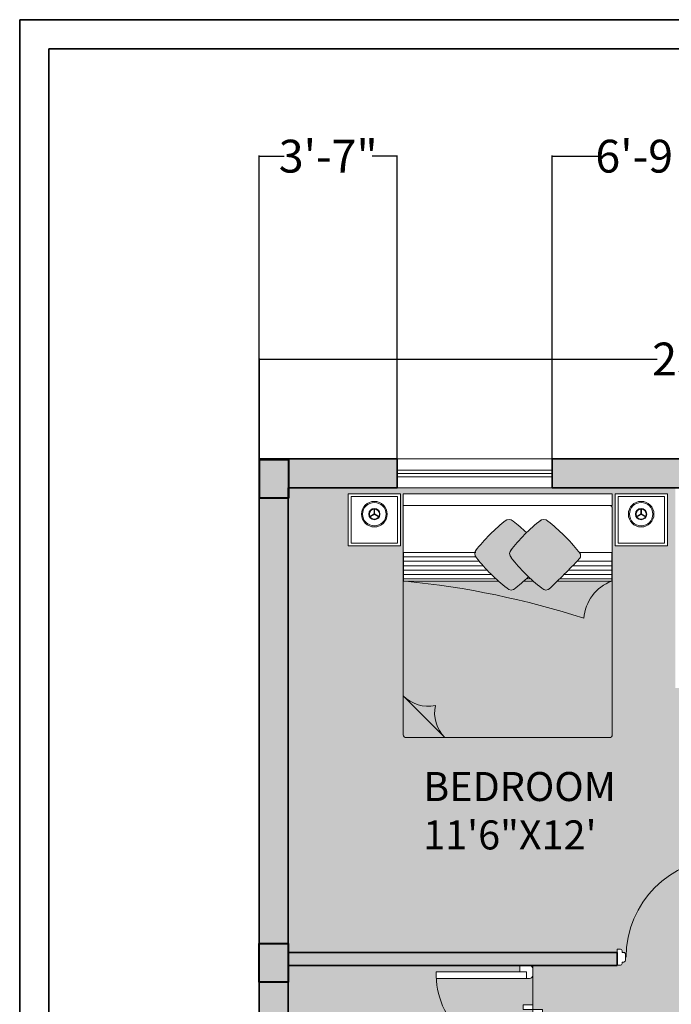
# Model space of a CAD drawing. Units: inches. Extents: x 1077 to 2505, y 1892 to 2728.
# Tile 25 of 26: x 1962 to 2164, y 2423 to 2728. Entities that reach past the tile are written whole.
import ezdxf

# ---------------------------------------------------------------- set-up
doc = ezdxf.new("R2010")
doc.units = ezdxf.units.IN
doc.linetypes.add('ACAD_ISO02W100', pattern=[15, 12, -3])
doc.layers.get('Defpoints').update_dxf_attribs({"color": 220, "linetype": 'ACAD_ISO02W100'})
for name, color, linetype, lineweight in [('00 FURNITURE', 15, 'Continuous', 15), ('A-ANNO-DIMS', 2, 'Continuous', 18), ('A-ANNO-TTLB', 7, 'Continuous', 35), ('A-AREA-IDEN', 7, 'Continuous', 18), ('A-COLS', 7, 'Continuous', 40), ('A-DOOR', 4, 'Continuous', 18), ('A-WALL-PATT', 7, 'Continuous', 9), ('A_FUR 1', 5, 'Continuous', 5), ('WALL', 7, 'Continuous', 35), ('WINDOW', 160, 'Continuous', 13)]:
    doc.layers.add(name, color=color, linetype=linetype, lineweight=lineweight)
doc.layers.add('A-FLOR-PATT', color=254, linetype='Continuous', lineweight=9, true_color=0xd7ebd2)
doc.layers.add('A-FURN-PATT', color=177, linetype='Continuous', lineweight=9, true_color=0x293189)
doc.styles.get("Standard").update_dxf_attribs({"font": 'arial.ttf'})
doc.dimstyles.get("Standard").update_dxf_attribs({"dimtxt": 10.18, "dimasz": 0.18, "dimexe": 0.18, "dimexo": 0.0625, "dimgap": 0.09, "dimtad": 0, "dimtih": 1, "dimtoh": 1, "dimdec": 0, "dimzin": 0, "dimdsep": 46, "dimlunit": 3, "dimtxsty": 'Standard', "dimcen": 0.09, "dimadec": 0, "dimazin": 0, "dimtfac": 1, "dimtdec": 0, "dimtofl": 0, "dimtmove": 0, "dimatfit": 3, "dimfxl": 1, "dimtolj": 1, "dimtzin": 0, "dimarcsym": 0})

# ---------------------------------------------------------------- blocks, each defined once
blk = doc.blocks.new('DDD')
at = {"layer": '00 FURNITURE'}
for p, q in [((-12579.77, -15859.53), (-12579.77, -15829.05)), ((-12578.77, -15859.53), (-12578.77, -15829.03)), ((-12612.02, -15857.03), (-12612.02, -15862.03)), ((-12611.02, -15857.03), (-12612.02, -15857.03)), ((-12610.52, -15858.03), (-12610.52, -15857.53)), ((-12577.52, -15858.03), (-12577.52, -15857.53)), ((-12577.02, -15857.03), (-12576.02, -15857.03)), ((-12576.02, -15857.03), (-12576.02, -15862.03)), ((-12610.52, -15861.53), (-12610.52, -15861.03)), ((-12578.77, -15859.53), (-12579.77, -15859.53)), ((-12577.52, -15861.53), (-12577.52, -15861.03)), ((-12612.02, -15862.03), (-12611.02, -15862.03)), ((-12576.02, -15862.03), (-12577.02, -15862.03))]:
    blk.add_line(p, q, dxfattribs=at)
for points in [[(-12610.52, -15861.03), (-12610.02, -15861.03, 0.414214), (-12609.52, -15860.53), (-12609.52, -15858.53, 0.414214), (-12610.02, -15858.03), (-12610.52, -15858.03)], [(-12577.52, -15861.03), (-12578.02, -15861.03, -0.414214), (-12578.52, -15860.53), (-12578.52, -15858.53, -0.414214), (-12578.02, -15858.03), (-12577.52, -15858.03)]]:
    blk.add_lwpolyline(points, format="xyb", dxfattribs=at)
for centre, radius, start, end in [((-12578.77, -15859.53), 30.5, 90, 180), ((-12611.02, -15857.53), 0.5, 0, 90), ((-12577.02, -15857.53), 0.5, 90, 180), ((-12611.02, -15861.53), 0.5, 270, 0), ((-12577.02, -15861.53), 0.5, 180, 270)]:
    blk.add_arc(centre, radius, start, end, dxfattribs=at)
blk = doc.blocks.new('ESTSET')
at = {"layer": 'A_FUR 1'}
for p, q in [((-10.44, 4.1), (-10.44, 32.1)), ((-8.44, 4.1), (-8.44, 32.1)), ((-36.44, 6.1), (-36.44, 3.1)), ((-34.44, 6.1), (-36.44, 6.1)), ((-34.44, 4.1), (-34.44, 6.1)), ((-34.44, 4.1), (-34.44, 6.1)), ((-32.44, 4.1), (-34.44, 4.1)), ((-32.44, 4.1), (-34.44, 4.1)), ((-32.44, 3.1), (-32.44, 4.1)), ((-10.44, 3.1), (-10.44, 4.1)), ((-10.44, 4.1), (-8.44, 4.1)), ((-10.44, 4.1), (-8.44, 4.1)), ((-8.44, 4.1), (-8.44, 6.1)), ((-8.44, 6.1), (-6.44, 6.1)), ((-8.44, 4.1), (-8.44, 6.1)), ((-6.44, 6.1), (-6.44, 3.1)), ((-6.44, 2.1), (-36.44, 2.1)), ((-35.44, 2.1), (-33.44, 2.1)), ((-7.44, 2.1), (-9.44, 2.1))]:
    blk.add_line(p, q, dxfattribs=at)
for points in [[(-21.44, 2.1), (-18.67, 2.1), (-18.67, 5.1), (-20.06, 5.1)], [(-20.06, 5.1), (-20.06, -0.91)], [(-21.44, 2.1), (-21.44, -0.91), (-20.06, -0.91)]]:
    blk.add_lwpolyline(points, dxfattribs=at)
for centre, radius, start, end in [((-8.91, 6.46), 25.64, 88.9606, 185.2816), ((-35.44, 3.1), 1, 180, 270), ((-33.44, 3.1), 1, 270, 0), ((-9.44, 3.1), 1, 180, 270), ((-7.44, 3.1), 1, 270, 0)]:
    blk.add_arc(centre, radius, start, end, dxfattribs=at)
blk = doc.blocks.new('RGWTG')
at = {"layer": '00 FURNITURE'}
for p, q in [((578.23, 3473.51), (577.36, 3475.01)), ((578.23, 3473.58), (577.36, 3472.08)), ((578.36, 3473.58), (577.49, 3475.09)), ((578.36, 3473.51), (577.49, 3472)), ((578.29, 3473.62), (580.03, 3473.62)), ((578.29, 3473.47), (580.03, 3473.47)), ((521.93, 3464.58), (509.03, 3451.68)), ((509.93, 3464.58), (566.4, 3464.58)), ((557.53, 3463.84), (557.53, 3464.49)), ((557.53, 3464.49), (566.4, 3464.49)), ((558.2, 3464.49), (558.2, 3435.82)), ((559.57, 3464.49), (559.57, 3437.25)), ((560.94, 3464.49), (560.94, 3438.58)), ((562.3, 3464.49), (562.3, 3439.83)), ((563.67, 3464.49), (563.67, 3440.99)), ((565.04, 3464.49), (565.04, 3442.08)), ((566.4, 3464.58), (580.98, 3464.58)), ((566.4, 3464.49), (566.4, 3442.08)), ((566.4, 3464.49), (566.4, 3463.84)), ((580.98, 3464.58), (580.98, 3416.72)), ((509.03, 3422.63), (509.03, 3463.68)), ((558.2, 3426.48), (558.2, 3425.04)), ((509.03, 3400.68), (509.03, 3422.63)), ((558.2, 3416.13), (558.2, 3399.95)), ((580.98, 3416.72), (580.98, 3400.68)), ((559.57, 3414.75), (559.57, 3399.95)), ((560.94, 3413.39), (560.94, 3399.95)), ((562.3, 3412.04), (562.3, 3399.95)), ((563.67, 3410.72), (563.67, 3399.95)), ((557.53, 3399.95), (557.53, 3400.6)), ((566.4, 3400.6), (566.4, 3399.95)), ((580.08, 3399.78), (509.93, 3399.78)), ((566.4, 3399.95), (557.53, 3399.95)), ((578.23, 3390.78), (577.36, 3392.29)), ((578.36, 3390.86), (577.49, 3392.36)), ((578.29, 3390.9), (580.03, 3390.9)), ((578.23, 3390.86), (577.36, 3389.36)), ((578.36, 3390.78), (577.49, 3389.28)), ((578.29, 3390.74), (580.03, 3390.74))]:
    blk.add_line(p, q, dxfattribs=at)
for points in [[(568.43, 3465.48), (584.63, 3465.48), (584.63, 3481.68), (568.43, 3481.68)], [(569.33, 3466.38), (583.73, 3466.38), (583.73, 3480.78), (569.33, 3480.78)], [(580.98, 3399.78), (584.63, 3399.78), (584.63, 3464.58), (580.98, 3464.58)], [(568.43, 3398.88), (584.63, 3398.88), (584.63, 3382.68), (568.43, 3382.68)], [(569.33, 3397.98), (583.73, 3397.98), (583.73, 3383.58), (569.33, 3383.58)]]:
    blk.add_lwpolyline(points, close=True, dxfattribs=at)
for points in [[(566.52, 3464.49), (557.53, 3464.49), (557.53, 3435.08)], [(557.53, 3427.21), (557.53, 3424.3)], [(557.53, 3416.82), (557.53, 3399.95), (566.4, 3399.95), (566.4, 3409.94)]]:
    blk.add_lwpolyline(points, dxfattribs=at)
for centre, radius in [((578.29, 3473.54), 3.97), ((578.29, 3473.54), 3.63), ((578.29, 3473.54), 1.74), ((578.29, 3473.54), 1.56), ((578.29, 3390.82), 3.97), ((578.29, 3390.82), 3.63), ((578.29, 3390.82), 1.74), ((578.29, 3390.82), 1.56)]:
    blk.add_circle(centre, radius, dxfattribs=at)
for centre, radius, start, end in [((509.93, 3463.68), 0.9, 90, 180), ((529.65, 3456.88), 10.9, 135.0361, 191.9278), ((290.56, 3490.52), 268.3, 342.2214, 354.2925), ((516.73, 3443.97), 10.9, 78.0722, 134.9639), ((598.15, 3399.01), 54.32, 127.931, 142.069), ((566.05, 3440.57), 1.82, 45, 135), ((533.58, 3399.31), 54.32, 37.931, 52.069), ((556.59, 3431.11), 1.82, 135, 225), ((598.15, 3388.23), 54.32, 127.931, 142.069), ((566.05, 3429.78), 1.82, 45, 135), ((533.58, 3388.53), 54.32, 37.931, 52.069), ((574.84, 3431.77), 1.82, 315, 45), ((597.87, 3463.6), 54.32, 217.931, 224.141), ((533.28, 3463.88), 54.32, 316.32, 322.069), ((556.59, 3420.33), 1.82, 135, 225), ((574.84, 3420.99), 1.82, 315, 45), ((765.33, 3619.75), 290.45, 223.6069, 226.2326), ((533.28, 3453.1), 54.32, 307.931, 322.069), ((565.44, 3411.05), 1.47, 225.9674, 326.8337), ((545.02, 3395.29), 13.35, 20.4224, 85.5825), ((509.93, 3400.68), 0.9, 180, 270), ((580.08, 3400.68), 0.9, 270, 0)]:
    blk.add_arc(centre, radius, start, end, dxfattribs=at)
blk = doc.blocks.new('C1')
h = blk.add_hatch(color=256)
h.dxf.hatch_style = 1
h.paths.add_polyline_path([(1668.56, 2445.41), (1677.56, 2445.41), (1677.56, 2457.41), (1668.56, 2457.41)])
for p, q in [((1668.56, 2457.41), (1677.56, 2457.41)), ((1668.56, 2445.41), (1668.56, 2457.41)), ((1677.56, 2457.41), (1677.56, 2445.41)), ((1677.56, 2445.41), (1668.56, 2445.41))]:
    blk.add_line(p, q)
blk = doc.blocks.new('*D18')
at = {"layer": 'A-ANNO-DIMS', "color": 0, "lineweight": -2, "transparency": 16777216}
for p, q in [((2035.96, 2592.42), (2035.96, 2623.29)), ((2036.14, 2623.11), (2159.23, 2623.11)), ((2317.64, 2623.11), (2194.55, 2623.11)), ((2317.82, 2592.42), (2317.82, 2623.29))]:
    blk.add_line(p, q, dxfattribs=at)
at = {"layer": 'A-ANNO-DIMS', "color": 0, "transparency": 16777216}
for points in [[(2036.14, 2623.14), (2036.14, 2623.08), (2035.96, 2623.11)], [(2317.64, 2623.14), (2317.64, 2623.08), (2317.82, 2623.11)]]:
    blk.add_solid(points, dxfattribs=at)
at = {"layer": 'Defpoints', "color": 0, "transparency": 16777216}
for p in [(2317.82, 2623.11), (2035.96, 2592.36), (2317.82, 2592.36)]:
    blk.add_point(p, dxfattribs=at)
at = {"layer": 'A-ANNO-DIMS', "color": 0, "transparency": 16777216, "insert": (2176.89, 2623.11), "char_height": 10.18, "attachment_point": 5}
blk.add_mtext('\\A1;23\'-6"', dxfattribs=at)
blk = doc.blocks.new('WINDOW-48-EXT')
for p, q in [((0, 48), (0, 0)), ((3.5, 48), (3.5, 0)), ((4.5, 48), (4.5, 0)), ((5.5, 48), (5.5, 0)), ((9, 0), (9, 48))]:
    blk.add_line(p, q)
blk = doc.blocks.new('SHEET-FRAME-RESIDENTIAL')
for points in [[(0, 830.04), (543.52, 830.04), (543.52, 0), (0, 0)], [(9, 821.04), (534.52, 821.04), (534.52, 9), (9, 9)]]:
    blk.add_lwpolyline(points, close=True)
blk = doc.blocks.new('*D73')
at = {"layer": 'A-ANNO-DIMS', "color": 0, "lineweight": -2, "transparency": 16777216}
for p, q in [((2035.85, 2592.2), (2035.85, 2686.17)), ((2036.03, 2685.99), (2043.62, 2685.99)), ((2078.45, 2685.99), (2070.86, 2685.99)), ((2078.63, 2592.2), (2078.63, 2686.17))]:
    blk.add_line(p, q, dxfattribs=at)
at = {"layer": 'A-ANNO-DIMS', "color": 0, "transparency": 16777216}
for points in [[(2036.03, 2686.02), (2036.03, 2685.96), (2035.85, 2685.99)], [(2078.45, 2686.02), (2078.45, 2685.96), (2078.63, 2685.99)]]:
    blk.add_solid(points, dxfattribs=at)
at = {"layer": 'Defpoints', "color": 0, "transparency": 16777216}
for p in [(2078.63, 2685.99), (2035.85, 2592.14), (2078.63, 2592.14)]:
    blk.add_point(p, dxfattribs=at)
at = {"layer": 'A-ANNO-DIMS', "color": 0, "transparency": 16777216, "insert": (2057.24, 2685.99), "char_height": 10.18, "attachment_point": 5}
blk.add_mtext('\\A1;3\'-7"', dxfattribs=at)
blk = doc.blocks.new('*D74')
at = {"layer": 'A-ANNO-DIMS', "color": 0, "lineweight": -2, "transparency": 16777216}
for p, q in [((2126.63, 2592.2), (2126.63, 2686.17)), ((2126.81, 2685.99), (2141.88, 2685.99)), ((2207.97, 2685.99), (2192.9, 2685.99)), ((2208.15, 2592.2), (2208.15, 2686.17))]:
    blk.add_line(p, q, dxfattribs=at)
at = {"layer": 'A-ANNO-DIMS', "color": 0, "transparency": 16777216}
for points in [[(2126.81, 2686.02), (2126.81, 2685.96), (2126.63, 2685.99)], [(2207.97, 2686.02), (2207.97, 2685.96), (2208.15, 2685.99)]]:
    blk.add_solid(points, dxfattribs=at)
at = {"layer": 'Defpoints', "color": 0, "transparency": 16777216}
for p in [(2208.15, 2685.99), (2126.63, 2592.14), (2208.15, 2592.14)]:
    blk.add_point(p, dxfattribs=at)
at = {"layer": 'A-ANNO-DIMS', "color": 0, "transparency": 16777216, "insert": (2167.39, 2685.99), "char_height": 10.18, "attachment_point": 5}
blk.add_mtext('\\A1;6\'-9 1/2"', dxfattribs=at)

msp = doc.modelspace()

# ---------------------------------------------------------------- hatches: boundary and pattern name
at = {"layer": 'A-FLOR-PATT', "transparency": 33554559}
h = msp.add_hatch(color=256, dxfattribs=at)
h.dxf.hatch_style = 1
h.paths.add_polyline_path([(2252.85, 2583.14), (2232.15, 2583.14), (2208.15, 2583.17), (2208.15, 2583.14), (2186.85, 2583.14), (2186.85, 2486.14), (2186.85, 2475.14), (2182.85, 2475.14), (2182.85, 2521.11), (2164.84, 2521.11), (2164.84, 2583.14), (2126.63, 2583.14), (2078.63, 2583.13), (2078.63, 2583.14), (2044.85, 2583.14), (2044.85, 2439.14), (2146.85, 2439.14), (2146.85, 2435.14), (2120.85, 2435.14), (2044.85, 2435.14), (2044.85, 2401), (2044.85, 2401), (2044.85, 2377), (2044.85, 2377), (2044.85, 2313.14), (2116.85, 2313.14), (2116.85, 2405.14), (2120.85, 2405.14), (2120.85, 2313.14), (2146.85, 2313.14), (2146.85, 2312.21), (2182.85, 2312.21), (2182.85, 2313.14), (2186.85, 2313.14), (2186.85, 2312.21), (2222.85, 2312.21), (2222.85, 2313.14), (2289.85, 2313.14), (2289.85, 2094.14), (2404.85, 2094.14), (2404.85, 2146.06), (2368.85, 2146.06), (2368.85, 2273.14), (2332.85, 2273.14), (2332.85, 2309.14), (2325.85, 2309.14), (2325.85, 2313.14), (2404.85, 2313.14), (2404.85, 2354.2), (2404.85, 2402.2), (2404.85, 2435.14), (2292.85, 2435.14), (2292.85, 2439.14), (2333.66, 2439.14), (2333.66, 2457.16), (2404.85, 2457.16), (2404.85, 2583.14), (2356.85, 2583.14), (2356.85, 2592.14), (2404.85, 2592.14), (2404.85, 2648.14), (2375.5, 2648.14), (2375.5, 2648.03), (2351.47, 2648.03), (2351.47, 2648.14), (2326.85, 2648.14), (2326.85, 2583.14), (2256.85, 2583.14), (2256.85, 2435.14), (2182.85, 2435.14), (2182.85, 2439.14), (2186.85, 2439.14), (2252.85, 2439.14), (2252.85, 2486.14), (2216.85, 2486.14), (2216.85, 2490.14), (2252.85, 2490.14)])
h.paths.add_polyline_path([(2214.97, 2488.05), (2212.97, 2488.05), (2212.97, 2487.05, 0.414214), (2213.97, 2486.05), (2201.97, 2486.05), (2201.97, 2483.04), (2200.58, 2483.04), (2200.58, 2486.05), (2187.97, 2486.05, -0.414214), (2186.97, 2487.05), (2186.97, 2490.05), (2188.97, 2490.05), (2188.97, 2516.05, -0.446908)], flags=16)
h.paths.add_polyline_path([(2162.4, 2565.16), (2146.2, 2565.16), (2146.2, 2581.36), (2162.4, 2581.36)], flags=16)
h.paths.add_polyline_path([(2161.5, 2566.06), (2147.1, 2566.06), (2147.1, 2580.46), (2161.5, 2580.46)], flags=0)
h.paths.add_polyline_path([(2145.3, 2506.66, -0.414214), (2144.4, 2505.76), (2122.45, 2505.76), (2081.4, 2505.76, -0.414214), (2080.5, 2506.66), (2080.5, 2563.14), (2080.5, 2577.72), (2080.5, 2581.36), (2145.3, 2581.36), (2145.3, 2577.72), (2144.4, 2577.72, -0.414214), (2145.3, 2576.82)], flags=16)
h.paths.add_polyline_path([(2150.3, 2575.03, -1), (2158.24, 2575.03, -1)], flags=0)
h.paths.add_polyline_path([(2150.64, 2575.03, -1), (2157.89, 2575.03, -1)], flags=0)
h.paths.add_polyline_path([(2180.11, 2468.19), (2180.11, 2437.69), (2180.36, 2436.69), (2180.36, 2437.69), (2179.11, 2437.69), (2179.11, 2468.17, 0.404641), (2149.61, 2437.69), (2149.36, 2436.69, -0.414214), (2148.86, 2436.19), (2148.36, 2436.19), (2148.36, 2435.69, -0.414214), (2147.86, 2435.19), (2146.86, 2435.19), (2146.86, 2440.19), (2147.86, 2440.19, -0.414214), (2148.36, 2439.69), (2148.36, 2439.19), (2148.86, 2439.19, -0.414214), (2149.36, 2438.69), (2149.61, 2437.69, -0.414214)], flags=16)
h.paths.add_polyline_path([(2145.14, 2554.26, 0.292232), (2136.49, 2542.78, 0.052719), (2081.25, 2554.26), (2080.6, 2554.26), (2080.6, 2563.14), (2081.25, 2563.14), (2102.73, 2563.14, -0.117785), (2103.09, 2563.91, -0.059418), (2112.19, 2573, -0.379859), (2114.6, 2572.86, -0.02509), (2118.73, 2569.3, -0.025935), (2122.97, 2573, -0.379859), (2125.38, 2572.86, -0.061767), (2134.84, 2563.41, -0.069393), (2135.14, 2563.14), (2145.14, 2563.14)], flags=0)
h.paths.add_polyline_path([(2120.79, 2554.26), (2117.88, 2554.26, -0.015371), (2115.33, 2552.11, -0.429576), (2112.69, 2552.04, -0.016036), (2110.01, 2554.26), (2080.6, 2554.26), (2080.6, 2560.4), (2104.1, 2560.4, 0.055344), (2112.69, 2552.04, 0.331768), (2114.84, 2551.72, 0.027343), (2119.32, 2555.62, 0.00919)], flags=0)
h.paths.add_polyline_path([(2152.88, 2574.32), (2154.19, 2575.07), (2154.19, 2576.58, 0.399698), (2152.71, 2575.03, 0.119004)], flags=0)
h.paths.add_polyline_path([(2152.53, 2575.03, -1), (2156, 2575.03, -1)], flags=0)
h.paths.add_polyline_path([(2154.27, 2574.94), (2154.34, 2574.98), (2154.34, 2575.07), (2154.3, 2575.09), (2154.23, 2574.96)], flags=0)
h.paths.add_polyline_path([(2259.6, 2468.17, -0.414214), (2290.1, 2437.67), (2290.35, 2438.67), (2290.1, 2437.67, 0.404641), (2260.6, 2468.15), (2260.6, 2437.67), (2259.35, 2437.67), (2259.35, 2436.67, -0.414214), (2258.85, 2436.17), (2258.35, 2436.17), (2258.35, 2435.67, -0.414214), (2257.85, 2435.17), (2256.85, 2435.17), (2256.85, 2440.17), (2257.85, 2440.17, -0.414214), (2258.35, 2439.67), (2258.35, 2439.17), (2258.85, 2439.17, -0.414214), (2259.35, 2438.67)], flags=16)
h.paths.add_polyline_path([(2327.48, 2541.19, -0.414214), (2328.38, 2542.09), (2384.85, 2542.09), (2399.43, 2542.09), (2403.08, 2542.09), (2403.08, 2477.29), (2399.43, 2477.29), (2399.43, 2478.19, -0.414214), (2398.53, 2477.29), (2328.38, 2477.29, -0.414214), (2327.48, 2478.19), (2327.48, 2500.14)], flags=16)
h.paths.add_polyline_path([(2340.38, 2542.09, 0.253465), (2337.43, 2532.13, 0.2538), (2327.47, 2529.17)], flags=16)
h.paths.add_polyline_path([(2080.5, 2518.67, 0.253465), (2090.46, 2515.72, 0.2538), (2093.42, 2505.75)], flags=16)
h.paths.add_polyline_path([(2327.09, 2584.7), (2327.09, 2587.7), (2329.09, 2587.7), (2329.09, 2613.7, -0.01951), (2331.09, 2613.66), (2331.09, 2585.7), (2331.09, 2584.7, -0.414214), (2330.09, 2583.7), (2328.09, 2583.7, -0.414214)], flags=16)
h.paths.add_polyline_path([(2239.78, 2404.11), (2252.36, 2404.11), (2252.36, 2405.72), (2239.78, 2405.72)], flags=16)
h.paths.add_polyline_path([(2237.26, 2403.16), (2237.26, 2395.8), (2237.82, 2395.8), (2237.82, 2402.03, -0.41429), (2238.38, 2402.59), (2253.79, 2402.59, -0.414213), (2254.35, 2402.03), (2254.35, 2395.8), (2254.91, 2395.8), (2254.91, 2403.16)], flags=16)
h.paths.add_polyline_path([(2120.69, 2434.12), (2120.69, 2432.12, -0.414214), (2119.69, 2431.12), (2118.69, 2431.12), (2090.73, 2431.12, 0.400854), (2116.69, 2407.02), (2116.69, 2407.12), (2118.69, 2407.12, -0.446908), (2090.69, 2433.12), (2116.69, 2433.12), (2116.69, 2435.12), (2119.69, 2435.12, -0.414214)], flags=16)
h.paths.add_polyline_path([(2262.11, 2404.11), (2274.69, 2404.11), (2274.69, 2405.72), (2262.11, 2405.72)], flags=16)
h.paths.add_polyline_path([(2259.59, 2403.16), (2262.11, 2404.11), (2274.69, 2404.11), (2277.24, 2403.16)], flags=16)
h.paths.add_polyline_path([(2289.58, 2389.14), (2289.58, 2376.57), (2291.19, 2376.57), (2291.19, 2389.14)], flags=16)
h.paths.add_polyline_path([(2288.62, 2391.67), (2281.15, 2391.67), (2281.15, 2391.11), (2287.5, 2391.11, -0.41429), (2288.06, 2390.54), (2288.06, 2375.14, -0.414237), (2287.5, 2374.58), (2281.15, 2374.58), (2281.15, 2374.01), (2288.62, 2374.01)], flags=16)
h.paths.add_polyline_path([(2274.69, 2357.14), (2274.69, 2355.52), (2276.22, 2355.52, 0.414236), (2277.24, 2356.54), (2277.24, 2358.09)], flags=16)
h.paths.add_polyline_path([(2252.36, 2357.14), (2252.36, 2355.52), (2253.89, 2355.52, 0.414235), (2254.91, 2356.54), (2254.91, 2358.09)], flags=16)
h.paths.add_polyline_path([(2224.02, 2376.03), (2222.41, 2376.03), (2222.41, 2374.5, 0.414235), (2223.43, 2373.48), (2224.98, 2373.48)], flags=16)
h.paths.add_polyline_path([(2276.68, 2365.45), (2276.68, 2359.22, -0.41419), (2276.12, 2358.66), (2260.71, 2358.66, -0.414137), (2260.15, 2359.22), (2260.15, 2365.45), (2254.35, 2365.45), (2254.35, 2359.22, -0.414189), (2253.79, 2358.66), (2238.38, 2358.66, -0.414137), (2237.82, 2359.22), (2237.82, 2365.45)], flags=16)
h.paths.add_polyline_path([(2079.6, 2565.16), (2063.4, 2565.16), (2063.4, 2581.36), (2079.6, 2581.36)], flags=16)
h.paths.add_polyline_path([(2078.7, 2566.06), (2064.3, 2566.06), (2064.3, 2580.46), (2078.7, 2580.46)], flags=0)
h.paths.add_polyline_path([(2339.31, 2583.7), (2339.31, 2586.71), (2340.7, 2586.71), (2340.7, 2583.7), (2342.09, 2583.7), (2342.09, 2580.7), (2340.7, 2580.7), (2340.7, 2583.7)], flags=16)
h.paths.add_polyline_path([(2123.69, 2421.51), (2123.69, 2420.12), (2120.69, 2420.12), (2120.69, 2421.51), (2117.68, 2421.51), (2117.68, 2422.89), (2120.69, 2422.89), (2120.69, 2421.51)], flags=16)
h.paths.add_polyline_path([(2067.57, 2575.03, -1), (2075.51, 2575.03, -1)], flags=0)
h.paths.add_polyline_path([(2067.92, 2575.03, -1), (2075.17, 2575.03, -1)], flags=0)
h.paths.add_polyline_path([(2070.16, 2574.32), (2071.47, 2575.07), (2071.47, 2576.58, 0.399698), (2069.99, 2575.03, 0.119004)], flags=0)
h.paths.add_polyline_path([(2069.81, 2575.03, -1), (2073.28, 2575.03, -1)], flags=0)
h.paths.add_polyline_path([(2071.54, 2574.94), (2071.62, 2574.89), (2071.62, 2574.98)], flags=0)
h.paths.add_polyline_path([(2364.5, 2486.1, 0.052719), (2375.98, 2541.34), (2375.98, 2541.99), (2384.85, 2541.99), (2384.85, 2541.34), (2384.85, 2519.86, -0.117785), (2385.62, 2519.51, -0.059418), (2394.72, 2510.41, -0.379859), (2394.58, 2507.99, -0.02509), (2391.01, 2503.87, -0.025935), (2394.72, 2499.62, -0.379859), (2394.58, 2497.21, -0.061767), (2385.12, 2487.75, -0.069393), (2384.85, 2487.45), (2384.85, 2477.45), (2375.98, 2477.45, 0.292232)], flags=0)
h.paths.add_polyline_path([(2373.75, 2509.9, -0.016036), (2375.98, 2512.58), (2375.98, 2541.99), (2382.12, 2541.99), (2382.12, 2518.49, 0.055344), (2373.75, 2509.9, 0.331768), (2373.44, 2507.75, 0.027343), (2377.33, 2503.27, 0.00919), (2375.98, 2501.8), (2375.98, 2504.71, -0.015371), (2373.82, 2507.26, -0.429576)], flags=0)
h.paths.add_polyline_path([(2356.95, 2631.48, -0.171636), (2360.13, 2636.99), (2360.13, 2639.35), (2356, 2639.35, -0.414214), (2355.01, 2640.34), (2355.01, 2646.64, -0.414214), (2356, 2647.62), (2372.14, 2647.62, -0.414214), (2373.13, 2646.64), (2373.13, 2640.34, -0.414214), (2372.14, 2639.35), (2368.01, 2639.35), (2368.01, 2636.99, -0.171636), (2371.2, 2631.48, -0.258205), (2366.63, 2620.45), (2361.51, 2620.45, -0.258205)], flags=16)
h.paths.add_polyline_path([(2358.52, 2631.48, -0.171636), (2361.71, 2636.99), (2366.43, 2636.99, -0.171636), (2369.62, 2631.48, -0.210384), (2366.67, 2622), (2361.47, 2622, -0.210384)], flags=0)
h.paths.add_polyline_path([(2386.88, 2542.99), (2386.88, 2559.19), (2403.08, 2559.19), (2403.08, 2542.99)], flags=16)
h.paths.add_polyline_path([(2387.78, 2543.89), (2387.78, 2558.29), (2402.18, 2558.29), (2402.18, 2543.89)], flags=0)
h.paths.add_polyline_path([(2392.77, 2551.05, -1), (2400.71, 2551.05, -1)], flags=0)
h.paths.add_polyline_path([(2393.11, 2551.05, -1), (2400.37, 2551.05, -1)], flags=0)
h.paths.add_polyline_path([(2386.88, 2476.39), (2403.08, 2476.39), (2403.08, 2460.19), (2386.88, 2460.19)], flags=16)
h.paths.add_polyline_path([(2398.48, 2550.97), (2398.3, 2550.97, -0.544606), (2396.03, 2549.66), (2395.94, 2549.51, 0.547962)], flags=0)
h.paths.add_polyline_path([(2387.78, 2475.49), (2402.18, 2475.49), (2402.18, 2461.09), (2387.78, 2461.09)], flags=0)
h.paths.add_polyline_path([(2396.79, 2551.12), (2396.74, 2551.2), (2396.7, 2551.12)], flags=0)
h.paths.add_polyline_path([(2400.71, 2468.32, -1), (2392.77, 2468.32, -1)], flags=0)
h.paths.add_polyline_path([(2400.37, 2468.32, -1), (2393.11, 2468.32, -1)], flags=0)
h.paths.add_polyline_path([(2398.48, 2468.25), (2398.3, 2468.25, -0.544606), (2396.03, 2466.94), (2395.94, 2466.78, 0.547962)], flags=0)
h.paths.add_polyline_path([(2396.79, 2468.4), (2396.74, 2468.48), (2396.7, 2468.4)], flags=0)
h.paths.add_polyline_path([(2292.64, 2341.23, -0.414214), (2323.14, 2310.73), (2323.39, 2311.73), (2323.14, 2310.73, 0.404641), (2293.64, 2341.21), (2293.64, 2310.73), (2292.39, 2310.73), (2292.39, 2309.73, -0.414214), (2291.89, 2309.23), (2291.39, 2309.23), (2291.39, 2308.73, -0.414214), (2290.89, 2308.23), (2289.89, 2308.23), (2289.89, 2313.23), (2290.89, 2313.23, -0.414214), (2291.39, 2312.73), (2291.39, 2312.23), (2291.89, 2312.23, -0.414214), (2292.39, 2311.73)], flags=16)
h.paths.add_polyline_path([(2389.45, 2641.69), (2392.75, 2641.69), (2392.75, 2641.87), (2389.45, 2641.87)], flags=16)
edge = h.paths.add_edge_path(flags=16)
edge.add_arc((2393.3, 2638.65), 0.183, 270, 360)
edge.add_line((2393.49, 2638.65), (2393.49, 2645.8))
edge.add_line((2393.49, 2645.8), (2395.61, 2645.8))
edge.add_line((2395.61, 2645.8), (2395.61, 2647.8))
edge.add_line((2395.61, 2647.8), (2390.57, 2647.8))
edge.add_line((2390.57, 2647.8), (2390.57, 2645.8))
edge.add_line((2390.57, 2645.8), (2392.19, 2645.8))
edge.add_line((2392.19, 2645.8), (2392.19, 2644.98))
edge.add_line((2392.19, 2644.98), (2391.02, 2644.98))
edge.add_line((2391.02, 2644.98), (2391.02, 2645.8))
edge.add_line((2391.02, 2645.8), (2390.57, 2645.8))
edge.add_line((2390.57, 2645.8), (2390.57, 2647.8))
edge.add_line((2390.57, 2647.8), (2395.61, 2647.8))
edge.add_line((2395.61, 2647.8), (2395.61, 2647.32))
edge.add_line((2395.61, 2647.32), (2397.95, 2647.56))
edge.add_line((2397.95, 2647.56), (2397.95, 2647.8))
edge.add_line((2397.95, 2647.8), (2398.81, 2647.8))
edge.add_line((2398.81, 2647.8), (2398.81, 2647.23))
edge.add_line((2398.81, 2647.23), (2398.63, 2645.77))
edge.add_ellipse((2398.41, 2644.93), major_axis=(-1.08, 0), ratio=0.790849, start_angle=180, end_angle=255.2976, ccw=False)
edge.add_line((2399.49, 2644.93), (2399.49, 2644.36))
edge.add_ellipse((2398.41, 2644.36), major_axis=(-1.08, 0), ratio=0.790849, start_angle=0, end_angle=180, ccw=False)
edge.add_line((2397.32, 2644.36), (2397.33, 2644.85))
edge.add_ellipse((2398.41, 2644.93), major_axis=(-1.08, 0), ratio=0.790849, start_angle=284.7024, end_angle=364.0401, ccw=False)
edge.add_line((2398.1, 2645.73), (2398.1, 2647.23))
edge.add_line((2398.1, 2647.23), (2397.95, 2647.23))
edge.add_line((2397.95, 2647.23), (2395.61, 2646.99))
edge.add_line((2395.61, 2646.99), (2395.61, 2645.8))
edge.add_line((2395.61, 2645.8), (2393.49, 2645.8))
edge.add_line((2393.49, 2645.8), (2393.49, 2638.46))
edge.add_line((2393.49, 2638.46), (2393.3, 2638.46))
h.paths.add_polyline_path([(2353.64, 2256.32, -0.292371), (2356.22, 2253.81, -0.085148), (2358.52, 2214.83, -0.01331), (2357.59, 2104.48, -0.379287), (2354.54, 2101.26, -0.0502), (2298.86, 2101.26, -0.379287), (2295.81, 2104.48, -0.01331), (2294.88, 2214.83, -0.086132), (2297.28, 2254.24, -0.295116), (2299.9, 2256.76, -0.114238)], flags=16)
h.paths.add_polyline_path([(2352.48, 2211.82, -0.355389), (2354.02, 2208.08), (2350.26, 2195.63, -0.398275), (2346.44, 2193.45, 0.113332), (2306.96, 2193.45, -0.398275), (2303.14, 2195.63), (2299.38, 2208.08, -0.355394), (2300.92, 2211.82, -0.265725)], flags=0)
h.paths.add_polyline_path([(2297.68, 2201.7), (2303.26, 2187.65), (2303.26, 2166.61), (2298.16, 2163.24)], flags=0)
h.paths.add_polyline_path([(2355.78, 2201.7), (2355.31, 2163.24), (2350.2, 2166.61), (2350.2, 2187.65)], flags=0)
h.paths.add_polyline_path([(2303.26, 2164.35), (2303.26, 2143.1), (2298.44, 2128.54), (2298.19, 2161.01)], flags=0)
h.paths.add_polyline_path([(2350.2, 2164.35), (2355.28, 2161.01), (2355.03, 2128.54), (2350.2, 2143.1)], flags=0)
h.paths.add_polyline_path([(2347.2, 2136.38), (2351.71, 2113.65, -0.090102), (2301.76, 2113.63), (2306.27, 2136.37, 0.036636)], flags=0)
h.paths.add_polyline_path([(2304.86, 2165.32), (2354.76, 2165.32), (2354.76, 2183.87), (2304.86, 2183.87)], flags=8)
h.paths.add_polyline_path([(2053.76, 2360.82), (2103.97, 2360.82), (2103.97, 2394.41), (2053.76, 2394.41)], flags=24)
h.paths.add_polyline_path([(2153.41, 2366.23), (2211.12, 2366.23), (2211.12, 2399.82), (2153.41, 2399.82)], flags=24)
h.paths.add_polyline_path([(2258.04, 2477.83), (2327.95, 2477.83), (2327.95, 2511.42), (2258.04, 2511.42)], flags=24)
h.paths.add_polyline_path([(2182.1, 2454.46), (2252.27, 2454.46), (2252.27, 2473), (2182.1, 2473)], flags=24)
h.paths.add_polyline_path([(2192.4, 2537.41), (2246.99, 2537.41), (2246.99, 2571), (2192.4, 2571)], flags=24)
h.paths.add_polyline_path([(2083.07, 2465.98), (2152.99, 2465.98), (2152.99, 2499.56), (2083.07, 2499.56)], flags=24)
at = {"layer": 'A-FURN-PATT', "transparency": 33554610}
h = msp.add_hatch(color=256, dxfattribs=at)
h.dxf.hatch_style = 1
h.paths.add_polyline_path([(2145.3, 2554.26), (2145.14, 2554.26, 0.292232), (2136.49, 2542.78, 0.052719), (2081.25, 2554.26), (2080.5, 2554.26), (2080.5, 2518.67, 0.253465), (2090.46, 2515.72, 0.253465), (2093.41, 2505.76), (2122.45, 2505.76), (2144.4, 2505.76, 0.414214), (2145.3, 2506.66)])
h.paths.add_polyline_path([(2080.5, 2518.67), (2080.5, 2506.66, 0.414214), (2081.4, 2505.76), (2093.41, 2505.76)], flags=17)
h.paths.add_polyline_path([(2134.84, 2563.41, 0.061767), (2125.38, 2572.86, 0.380465), (2122.96, 2573.01, 0.059418), (2113.87, 2563.91, 0.379859), (2114.01, 2561.49, 0.061767), (2123.47, 2552.04, 0.334836), (2125.64, 2551.73, 0.011497), (2135.1, 2561.16, 0.468078)])
h.paths.add_polyline_path([(2113.87, 2563.91, -0.033431), (2118.73, 2569.3, 0.025099), (2114.6, 2572.86, 0.380465), (2112.18, 2573.01, 0.059418), (2103.09, 2563.91, 0.379859), (2103.23, 2561.49, 0.061767), (2112.69, 2552.04, 0.331768), (2114.84, 2551.72, 0.027343), (2119.32, 2555.62, -0.036481), (2114.01, 2561.49, -0.379859)])
h.paths.add_polyline_path([(2145.14, 2554.26), (2128.27, 2554.26, -0.003141), (2125.64, 2551.73, -0.334836), (2123.47, 2552.04, -0.016036), (2120.79, 2554.26), (2117.88, 2554.26, -0.015371), (2115.33, 2552.11, -0.429576), (2112.69, 2552.04, -0.016036), (2110.01, 2554.26), (2081.25, 2554.26, -0.052719), (2136.49, 2542.78, -0.292232)], flags=17)
at = {"layer": 'A-WALL-PATT', "transparency": 33554585}
h = msp.add_hatch(color=256, dxfattribs=at)
h.dxf.hatch_style = 1
h.paths.add_polyline_path([(2044.85, 2429.98), (2035.85, 2429.98), (2035.85, 2401), (2044.85, 2401)])
h.paths.add_polyline_path([(2044.85, 2377), (2035.85, 2377), (2035.85, 2317.47), (2044.85, 2317.47)])
h.paths.add_polyline_path([(2085.45, 2159.14), (2044.85, 2159.14), (2044.85, 2225.64), (2035.85, 2225.64), (2035.85, 2106.16), (2044.85, 2106.16), (2044.85, 2150.14), (2085.45, 2150.14)])
h.paths.add_polyline_path([(2289.85, 2103.14), (2044.85, 2103.14), (2044.85, 2106.16), (2035.85, 2106.16), (2035.85, 2094.14), (2289.85, 2094.14)])
h.paths.add_polyline_path([(2413.85, 2354.2), (2404.85, 2354.2), (2404.85, 2354.2), (2404.85, 2313.14), (2325.85, 2313.14), (2325.85, 2309.14), (2404.85, 2309.14), (2404.85, 2094.14), (2413.85, 2094.14)])
h.paths.add_polyline_path([(2413.85, 2431.09), (2404.85, 2431.09), (2404.85, 2402.2), (2413.85, 2402.2)])
h.paths.add_polyline_path([(2404.85, 2439.14), (2292.85, 2439.14), (2292.85, 2435.14), (2404.85, 2435.14)])
h.paths.add_polyline_path([(2413.85, 2580.36), (2404.85, 2580.36), (2404.85, 2457.16), (2404.87, 2457.16), (2404.87, 2443.09), (2413.85, 2443.09)])
h.paths.add_polyline_path([(2413.85, 2645.09), (2404.85, 2645.09), (2404.85, 2592.36), (2413.85, 2592.36)])
h.paths.add_polyline_path([(2413.85, 2645.09), (2404.85, 2645.09), (2404.85, 2648.14), (2375.5, 2648.14), (2375.5, 2648.03), (2351.5, 2648.03), (2351.5, 2657.03), (2375.47, 2657.03), (2375.47, 2657.14), (2413.85, 2657.14)])
h.paths.add_polyline_path([(2351.47, 2657.14), (2326.92, 2657.14), (2326.92, 2648.14), (2351.47, 2648.14)])
h.paths.add_polyline_path([(2078.63, 2583.14), (2044.92, 2583.14), (2044.92, 2580.01), (2035.92, 2580.01), (2035.92, 2592.14), (2078.63, 2592.14)])
h.paths.add_polyline_path([(2180.39, 2592.14), (2126.63, 2592.14), (2126.63, 2583.14), (2180.39, 2583.14)])
h.paths.add_polyline_path([(2232.16, 2592.17), (2232.16, 2583.17), (2208.16, 2583.17), (2208.15, 2583.17), (2208.15, 2583.14), (2189.39, 2583.14), (2189.39, 2579.98), (2180.39, 2579.98), (2180.39, 2592.14), (2208.15, 2592.14), (2208.16, 2592.14), (2208.16, 2592.17)])
h.paths.add_polyline_path([(2250.27, 2592.14), (2232.16, 2592.14), (2232.16, 2583.14), (2250.27, 2583.14)], flags=17)
h.paths.add_polyline_path([(2326.85, 2648.14), (2326.92, 2657.14), (2317.85, 2657.14), (2317.85, 2592.14), (2250.27, 2592.14), (2250.27, 2583.14), (2252.85, 2583.14), (2252.85, 2490.14), (2216.85, 2490.14), (2216.85, 2486.14), (2252.85, 2486.14), (2252.85, 2439.14), (2186.85, 2439.14), (2182.85, 2439.14), (2182.85, 2435.14), (2256.85, 2435.14), (2256.85, 2583.14), (2326.85, 2583.14)])
h.paths.add_polyline_path([(2044.85, 2580.01), (2035.85, 2580.01), (2035.85, 2441.98), (2044.85, 2441.98)])
at = {"layer": 'A-WALL-PATT', "transparency": 33554559}
h = msp.add_hatch(color=256, dxfattribs=at)
h.dxf.hatch_style = 1
h.paths.add_polyline_path([(2146.85, 2439.14), (2044.78, 2439.14), (2044.78, 2435.14), (2120.85, 2435.14), (2146.85, 2435.14)])
h.paths.add_polyline_path([(2186.85, 2579.98), (2182.85, 2579.98), (2182.85, 2475.14), (2186.85, 2475.14), (2186.85, 2486.14)])
h.paths.add_polyline_path([(2404.83, 2592.14), (2356.85, 2592.14), (2356.85, 2587.7), (2357.09, 2587.7), (2357.09, 2584.7, -0.178139), (2356.85, 2584.05), (2356.85, 2583.14), (2404.83, 2583.14)])
h.paths.add_polyline_path([(2186.85, 2159.14), (2133.45, 2159.14), (2133.45, 2150.14), (2186.85, 2150.14)])

# ---------------------------------------------------------------- linework, layer by layer
at = {"layer": 'WALL'}
for p, q in [((2035.85, 2592.14), (2078.63, 2592.14)), ((2035.85, 2401), (2035.85, 2592.14)), ((2078.63, 2583.14), (2078.63, 2592.14)), ((2126.63, 2592.14), (2208.15, 2592.14)), ((2126.63, 2583.14), (2126.63, 2592.14)), ((2044.85, 2583.14), (2078.63, 2583.14)), ((2044.85, 2439.14), (2044.85, 2583.14)), ((2126.63, 2583.14), (2182.85, 2583.14)), ((2044.85, 2439.14), (2146.85, 2439.14)), ((2146.85, 2435.14), (2146.85, 2439.14)), ((2044.85, 2435.14), (2120.85, 2435.14)), ((2044.85, 2401), (2044.85, 2435.14)), ((2120.85, 2435.14), (2146.85, 2435.14))]:
    msp.add_line(p, q, dxfattribs=at)

# ---------------------------------------------------------------- block references
at = {"layer": '00 FURNITURE', "rotation": 89.99999999999999}
msp.add_blockref('RGWTG', (5545.09, 1996.73), dxfattribs=at)
at = {"layer": 'A-ANNO-TTLB'}
msp.add_blockref('SHEET-FRAME-RESIDENTIAL', (1961.57, 1898.25), dxfattribs=at)
at = {"layer": 'A-COLS'}
for p in [(367.37, 134.6), (367.22, -15.43)]:
    msp.add_blockref('C1', p, dxfattribs=at)
at = {"layer": 'A-DOOR'}
msp.add_blockref('DDD', (14758.89, 18297.22), dxfattribs=at)
at = {"layer": 'A-DOOR', "rotation": 90.00000000000003}
msp.add_blockref('ESTSET', (2122.78, 2441.57), dxfattribs=at)
at = {"layer": 'WINDOW', "rotation": 90.00000000000031}
msp.add_blockref('WINDOW-48-EXT', (2126.64, 2583.13), dxfattribs=at)

# ---------------------------------------------------------------- texts
at = {"layer": 'A-AREA-IDEN', "insert": (2086.69, 2495.09), "char_height": 9, "attachment_point": 1}
msp.add_mtext_dynamic_manual_height_columns('BEDROOM\\P11\'6"X12\'', width=128.1076, gutter_width=12.5, heights=[0], dxfattribs=at)

# ---------------------------------------------------------------- dimensions: what is measured, and where the dimension line sits
at = {"layer": 'A-ANNO-DIMS'}
for base, p1, p2, override, picture, middle in [((2208.15, 2685.99), (2126.63, 2592.14), (2208.15, 2592.14), {"dimdec": 1, "dimlfac": 1, "dimrnd": 0, "dimzin": 1, "dimdsep": 46, "dimlunit": 4, "dimfrac": 2}, '*D74', (2167.39, 2685.99)), ((2078.63, 2685.99), (2035.85, 2592.14), (2078.63, 2592.14), {"dimdec": 1, "dimlfac": 1, "dimrnd": 0, "dimzin": 1, "dimdsep": 46, "dimlunit": 4, "dimfrac": 2}, '*D73', (2057.24, 2685.99)), ((2317.82, 2623.11), (2035.96, 2592.36), (2317.82, 2592.36), {"dimclrd": 0, "dimclre": 0, "dimclrt": 0}, '*D18', (2176.89, 2623.11))]:
    dim = msp.add_linear_dim(base=base, p1=p1, p2=p2, dimstyle='Standard', override=override, dxfattribs=at)
    dim.commit()
    dim.dimension.update_dxf_attribs({"geometry": picture, "text_midpoint": middle})

doc.saveas('drawing.dxf')
